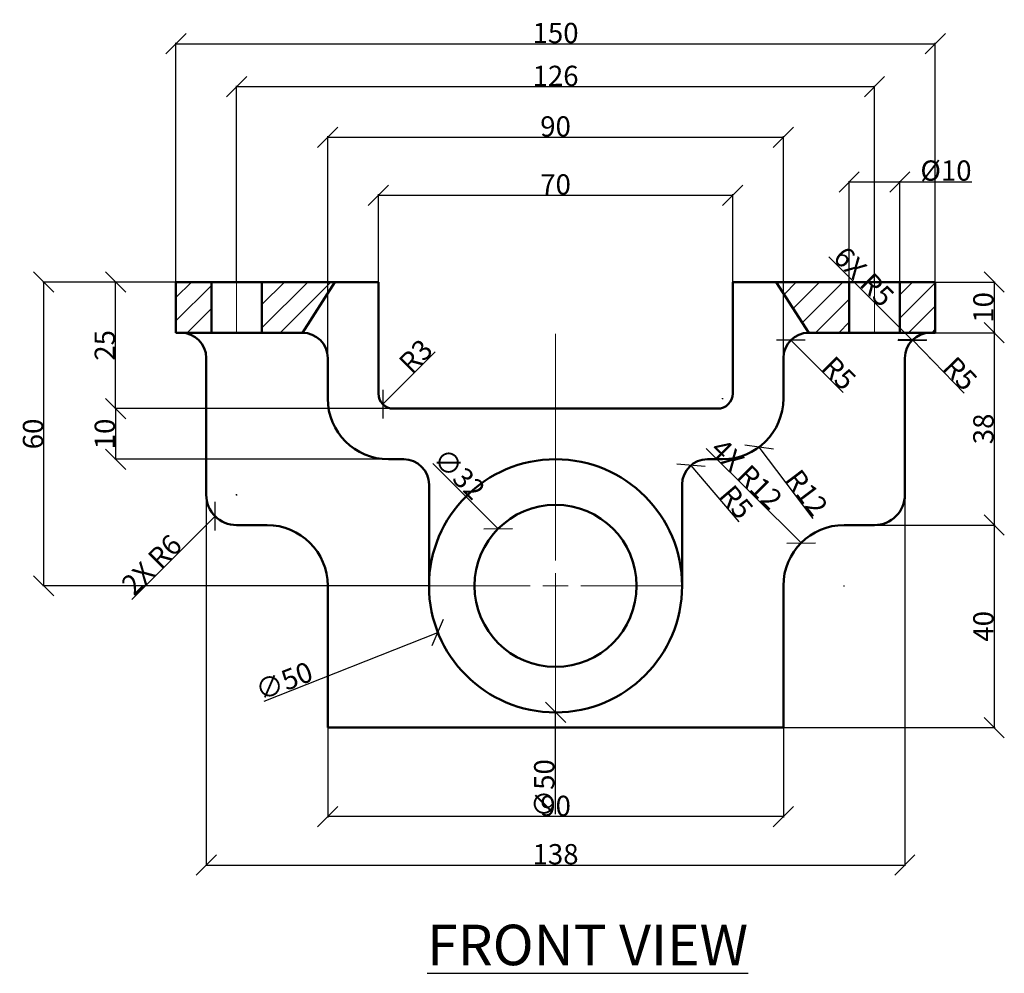
# Model space of a CAD drawing. Units: millimetres. Extents: x 113 to 503, y 39 to 409.
# Tile 2 of 3: x 113 to 307, y 221 to 409. Entities that reach past the tile are written whole.
import ezdxf

# ---------------------------------------------------------------- set-up
doc = ezdxf.new("R2010")
doc.units = ezdxf.units.MM
doc.header["$MEASUREMENT"] = 0
doc.linetypes.add('CENTER', pattern=[50.8, 31.75, -6.35, 6.35, -6.35])
for name, color, linetype, lineweight in [('M-CNTR', 1, 'CENTER', 18), ('M-DIMS', 2, 'Continuous', 25), ('M-HATC', 8, 'Continuous', 18), ('M-OUTL', 7, 'Continuous', 50), ('M-TEXT', 3, 'Continuous', 25)]:
    doc.layers.add(name, color=color, linetype=linetype, lineweight=lineweight)
doc.styles.get("Standard").update_dxf_attribs({"font": 'arial.ttf'})
doc.dimstyles.get("Standard").update_dxf_attribs({"dimtxt": 4, "dimasz": 4, "dimexe": 0.18, "dimexo": 0.0625, "dimgap": 0.09, "dimtad": 1, "dimdec": 0, "dimzin": 0, "dimdsep": 46, "dimtxsty": 'Standard', "dimblk": 'OBLIQUE', "dimcen": 0.09, "dimclre": 251, "dimadec": 0, "dimazin": 0, "dimtfac": 1, "dimtdec": 0, "dimtofl": 0, "dimtmove": 0, "dimatfit": 3, "dimfxl": 1, "dimtolj": 1, "dimtzin": 0, "dimarcsym": 0})
pattern_1 = [(45, (99.4996, 254.7123), (-2.298097, 2.298097), [])]

# ---------------------------------------------------------------- blocks, each defined once
blk = doc.blocks.new('*U2')
at = {"layer": 'M-CNTR', "color": 0, "transparency": 16777216}
for p, q in [((0, 5), (0, 25.12)), ((-25.12, 0), (-5, 0)), ((5, 0), (25.12, 0)), ((0, -25.12), (0, -5))]:
    blk.add_line(p, q, dxfattribs=at)
at = {"layer": 'M-CNTR', "color": 0, "linetype": 'Continuous', "transparency": 16777216}
for p, q in [((0, -2.5), (0, 2.5)), ((-2.5, 0), (2.5, 0))]:
    blk.add_line(p, q, dxfattribs=at)
blk = doc.blocks.new('_Oblique')
at = {"color": 0, "linetype": 'ByBlock', "lineweight": -2}
blk.add_line((-0.5, -0.5), (0.5, 0.5), dxfattribs=at)
blk = doc.blocks.new('*D3')
at = {"layer": 'Defpoints', "color": 0, "transparency": 16777216}
for p in [(253.81, 374.39), (183.81, 357.23), (253.81, 357.23)]:
    blk.add_point(p, dxfattribs=at)
at = {"layer": 'M-DIMS', "color": 0, "lineweight": -2, "transparency": 16777216}
for p, q in [((183.81, 357.29), (183.81, 374.57)), ((183.81, 374.39), (253.81, 374.39)), ((253.81, 357.29), (253.81, 374.57))]:
    blk.add_line(p, q, dxfattribs=at)
at = {"layer": 'M-DIMS', "color": 0, "lineweight": -2, "transparency": 16777216, "xscale": 4, "yscale": 4, "zscale": 4, "rotation": 180}
blk.add_blockref('_Oblique', (183.81, 374.39), dxfattribs=at)
at = {"layer": 'M-DIMS', "color": 0, "lineweight": -2, "transparency": 16777216, "xscale": 4, "yscale": 4, "zscale": 4}
blk.add_blockref('_Oblique', (253.81, 374.39), dxfattribs=at)
at = {"layer": 'M-DIMS', "color": 0, "transparency": 16777216, "insert": (218.81, 376.52), "char_height": 4, "attachment_point": 5}
blk.add_mtext('\\A1;70', dxfattribs=at)
blk = doc.blocks.new('*D4')
at = {"layer": 'Defpoints', "color": 0, "transparency": 16777216}
for p in [(263.81, 385.85), (173.81, 342.23), (263.81, 342.23)]:
    blk.add_point(p, dxfattribs=at)
at = {"layer": 'M-DIMS', "color": 0, "lineweight": -2, "transparency": 16777216}
for p, q in [((173.81, 342.29), (173.81, 386.03)), ((173.81, 385.85), (263.81, 385.85)), ((263.81, 342.29), (263.81, 386.03))]:
    blk.add_line(p, q, dxfattribs=at)
at = {"layer": 'M-DIMS', "color": 0, "lineweight": -2, "transparency": 16777216, "xscale": 4, "yscale": 4, "zscale": 4, "rotation": 180}
blk.add_blockref('_Oblique', (173.81, 385.85), dxfattribs=at)
at = {"layer": 'M-DIMS', "color": 0, "lineweight": -2, "transparency": 16777216, "xscale": 4, "yscale": 4, "zscale": 4}
blk.add_blockref('_Oblique', (263.81, 385.85), dxfattribs=at)
at = {"layer": 'M-DIMS', "color": 0, "transparency": 16777216, "insert": (218.81, 387.98), "char_height": 4, "attachment_point": 5}
blk.add_mtext('\\A1;90', dxfattribs=at)
blk = doc.blocks.new('*D5')
at = {"layer": 'Defpoints', "color": 0, "transparency": 16777216}
for p in [(281.81, 395.84), (155.81, 357.23), (281.81, 357.23)]:
    blk.add_point(p, dxfattribs=at)
at = {"layer": 'M-DIMS', "color": 0, "lineweight": -2, "transparency": 16777216}
for p, q in [((155.81, 357.29), (155.81, 396.02)), ((155.81, 395.84), (281.81, 395.84)), ((281.81, 357.29), (281.81, 396.02))]:
    blk.add_line(p, q, dxfattribs=at)
at = {"layer": 'M-DIMS', "color": 0, "lineweight": -2, "transparency": 16777216, "xscale": 4, "yscale": 4, "zscale": 4, "rotation": 180}
blk.add_blockref('_Oblique', (155.81, 395.84), dxfattribs=at)
at = {"layer": 'M-DIMS', "color": 0, "lineweight": -2, "transparency": 16777216, "xscale": 4, "yscale": 4, "zscale": 4}
blk.add_blockref('_Oblique', (281.81, 395.84), dxfattribs=at)
at = {"layer": 'M-DIMS', "color": 0, "transparency": 16777216, "insert": (218.81, 397.97), "char_height": 4, "attachment_point": 5}
blk.add_mtext('\\A1;126', dxfattribs=at)
blk = doc.blocks.new('*D6')
at = {"layer": 'Defpoints', "color": 0, "transparency": 16777216}
for p in [(293.81, 404.31), (143.81, 357.23), (293.81, 357.23)]:
    blk.add_point(p, dxfattribs=at)
at = {"layer": 'M-DIMS', "color": 0, "lineweight": -2, "transparency": 16777216}
for p, q in [((143.81, 357.29), (143.81, 404.49)), ((143.81, 404.31), (293.81, 404.31)), ((293.81, 357.29), (293.81, 404.49))]:
    blk.add_line(p, q, dxfattribs=at)
at = {"layer": 'M-DIMS', "color": 0, "lineweight": -2, "transparency": 16777216, "xscale": 4, "yscale": 4, "zscale": 4, "rotation": 180}
blk.add_blockref('_Oblique', (143.81, 404.31), dxfattribs=at)
at = {"layer": 'M-DIMS', "color": 0, "lineweight": -2, "transparency": 16777216, "xscale": 4, "yscale": 4, "zscale": 4}
blk.add_blockref('_Oblique', (293.81, 404.31), dxfattribs=at)
at = {"layer": 'M-DIMS', "color": 0, "transparency": 16777216, "insert": (218.81, 406.44), "char_height": 4, "attachment_point": 5}
blk.add_mtext('\\A1;150', dxfattribs=at)
blk = doc.blocks.new('*D7')
at = {"layer": 'Defpoints', "color": 0, "transparency": 16777216}
for p in [(286.81, 377.02), (276.81, 357.23), (286.81, 357.23)]:
    blk.add_point(p, dxfattribs=at)
at = {"layer": 'M-DIMS', "color": 0, "lineweight": -2, "transparency": 16777216}
for p, q in [((276.81, 357.29), (276.81, 377.2)), ((276.81, 377.02), (286.81, 377.02)), ((286.81, 357.29), (286.81, 377.2)), ((286.81, 377.02), (301.06, 377.02))]:
    blk.add_line(p, q, dxfattribs=at)
at = {"layer": 'M-DIMS', "color": 0, "lineweight": -2, "transparency": 16777216, "xscale": 4, "yscale": 4, "zscale": 4, "rotation": 180}
blk.add_blockref('_Oblique', (276.81, 377.02), dxfattribs=at)
at = {"layer": 'M-DIMS', "color": 0, "lineweight": -2, "transparency": 16777216, "xscale": 4, "yscale": 4, "zscale": 4}
blk.add_blockref('_Oblique', (286.81, 377.02), dxfattribs=at)
at = {"layer": 'M-DIMS', "color": 0, "transparency": 16777216, "insert": (295.93, 379.26), "char_height": 4, "attachment_point": 5}
blk.add_mtext('\\A1;%%C10', dxfattribs=at)
blk = doc.blocks.new('*D8')
at = {"layer": 'Defpoints', "color": 0, "transparency": 16777216}
for p in [(117.71, 357.23), (143.81, 357.23), (193.69, 297.23)]:
    blk.add_point(p, dxfattribs=at)
at = {"layer": 'M-DIMS', "color": 0, "lineweight": -2, "transparency": 16777216}
for p, q in [((143.75, 357.23), (117.53, 357.23)), ((117.71, 297.23), (117.71, 357.23)), ((193.63, 297.23), (117.53, 297.23))]:
    blk.add_line(p, q, dxfattribs=at)
at = {"layer": 'M-DIMS', "color": 0, "lineweight": -2, "transparency": 16777216, "xscale": 4, "yscale": 4, "zscale": 4}
for p, rotation in [((117.71, 357.23), 90), ((117.71, 297.23), 270)]:
    blk.add_blockref('_Oblique', p, dxfattribs=dict(at, rotation=rotation))
at = {"layer": 'M-DIMS', "color": 0, "transparency": 16777216, "insert": (115.58, 327.23), "char_height": 4, "attachment_point": 5, "rotation": 90}
blk.add_mtext('\\A1;60', dxfattribs=at)
blk = doc.blocks.new('*D9')
at = {"layer": 'Defpoints', "color": 0, "transparency": 16777216}
for p in [(131.9, 357.23), (143.81, 357.23), (186.81, 332.23)]:
    blk.add_point(p, dxfattribs=at)
at = {"layer": 'M-DIMS', "color": 0, "lineweight": -2, "transparency": 16777216}
for p, q in [((143.75, 357.23), (131.72, 357.23)), ((131.9, 332.23), (131.9, 357.23)), ((186.75, 332.23), (131.72, 332.23))]:
    blk.add_line(p, q, dxfattribs=at)
at = {"layer": 'M-DIMS', "color": 0, "lineweight": -2, "transparency": 16777216, "xscale": 4, "yscale": 4, "zscale": 4}
for p, rotation in [((131.9, 357.23), 90), ((131.9, 332.23), 270)]:
    blk.add_blockref('_Oblique', p, dxfattribs=dict(at, rotation=rotation))
at = {"layer": 'M-DIMS', "color": 0, "transparency": 16777216, "insert": (129.76, 344.73), "char_height": 4, "attachment_point": 5, "rotation": 90}
blk.add_mtext('\\A1;25', dxfattribs=at)
blk = doc.blocks.new('*D10')
at = {"layer": 'Defpoints', "color": 0, "transparency": 16777216}
for p in [(186.81, 332.23), (131.9, 322.23), (187.31, 322.23)]:
    blk.add_point(p, dxfattribs=at)
at = {"layer": 'M-DIMS', "color": 0, "lineweight": -2, "transparency": 16777216}
for p, q in [((186.75, 332.23), (131.72, 332.23)), ((131.9, 332.23), (131.9, 322.23)), ((187.25, 322.23), (131.72, 322.23))]:
    blk.add_line(p, q, dxfattribs=at)
at = {"layer": 'M-DIMS', "color": 0, "lineweight": -2, "transparency": 16777216, "xscale": 4, "yscale": 4, "zscale": 4}
for p, rotation in [((131.9, 332.23), 90), ((131.9, 322.23), 270)]:
    blk.add_blockref('_Oblique', p, dxfattribs=dict(at, rotation=rotation))
at = {"layer": 'M-DIMS', "color": 0, "transparency": 16777216, "insert": (129.76, 327.23), "char_height": 4, "attachment_point": 5, "rotation": 90}
blk.add_mtext('\\A1;10', dxfattribs=at)
blk = doc.blocks.new('*D11')
at = {"layer": 'Defpoints', "color": 0, "transparency": 16777216}
for p in [(293.81, 357.23), (293.81, 347.23), (305.46, 347.23)]:
    blk.add_point(p, dxfattribs=at)
at = {"layer": 'M-DIMS', "color": 0, "lineweight": -2, "transparency": 16777216}
for p, q in [((293.87, 357.23), (305.64, 357.23)), ((305.46, 357.23), (305.46, 347.23)), ((293.87, 347.23), (305.64, 347.23))]:
    blk.add_line(p, q, dxfattribs=at)
at = {"layer": 'M-DIMS', "color": 0, "lineweight": -2, "transparency": 16777216, "xscale": 4, "yscale": 4, "zscale": 4}
for p, rotation in [((305.46, 357.23), 90), ((305.46, 347.23), 270)]:
    blk.add_blockref('_Oblique', p, dxfattribs=dict(at, rotation=rotation))
at = {"layer": 'M-DIMS', "color": 0, "transparency": 16777216, "insert": (303.32, 352.23), "char_height": 4, "attachment_point": 5, "rotation": 90}
blk.add_mtext('\\A1;10', dxfattribs=at)
blk = doc.blocks.new('*D12')
at = {"layer": 'Defpoints', "color": 0, "transparency": 16777216}
for p in [(293.81, 347.23), (278.81, 309.23), (305.46, 309.23)]:
    blk.add_point(p, dxfattribs=at)
at = {"layer": 'M-DIMS', "color": 0, "lineweight": -2, "transparency": 16777216}
for p, q in [((293.87, 347.23), (305.64, 347.23)), ((305.46, 347.23), (305.46, 309.23)), ((278.87, 309.23), (305.64, 309.23))]:
    blk.add_line(p, q, dxfattribs=at)
at = {"layer": 'M-DIMS', "color": 0, "lineweight": -2, "transparency": 16777216, "xscale": 4, "yscale": 4, "zscale": 4}
for p, rotation in [((305.46, 347.23), 90), ((305.46, 309.23), 270)]:
    blk.add_blockref('_Oblique', p, dxfattribs=dict(at, rotation=rotation))
at = {"layer": 'M-DIMS', "color": 0, "transparency": 16777216, "insert": (303.32, 328.23), "char_height": 4, "attachment_point": 5, "rotation": 90}
blk.add_mtext('\\A1;38', dxfattribs=at)
blk = doc.blocks.new('*D13')
at = {"layer": 'Defpoints', "color": 0, "transparency": 16777216}
for p in [(278.81, 309.23), (263.81, 269.23), (305.46, 269.23)]:
    blk.add_point(p, dxfattribs=at)
at = {"layer": 'M-DIMS', "color": 0, "lineweight": -2, "transparency": 16777216}
for p, q in [((278.87, 309.23), (305.64, 309.23)), ((305.46, 309.23), (305.46, 269.23)), ((263.87, 269.23), (305.64, 269.23))]:
    blk.add_line(p, q, dxfattribs=at)
at = {"layer": 'M-DIMS', "color": 0, "lineweight": -2, "transparency": 16777216, "xscale": 4, "yscale": 4, "zscale": 4}
for p, rotation in [((305.46, 309.23), 90), ((305.46, 269.23), 270)]:
    blk.add_blockref('_Oblique', p, dxfattribs=dict(at, rotation=rotation))
at = {"layer": 'M-DIMS', "color": 0, "transparency": 16777216, "insert": (303.32, 289.23), "char_height": 4, "attachment_point": 5, "rotation": 90}
blk.add_mtext('\\A1;40', dxfattribs=at)
blk = doc.blocks.new('*D14')
at = {"layer": 'Defpoints', "color": 0, "transparency": 16777216}
for p in [(173.81, 269.23), (263.81, 269.23), (173.81, 251.63)]:
    blk.add_point(p, dxfattribs=at)
at = {"layer": 'M-DIMS', "color": 0, "lineweight": -2, "transparency": 16777216}
for p, q in [((173.81, 269.16), (173.81, 251.45)), ((263.81, 269.16), (263.81, 251.45)), ((263.81, 251.63), (173.81, 251.63))]:
    blk.add_line(p, q, dxfattribs=at)
at = {"layer": 'M-DIMS', "color": 0, "lineweight": -2, "transparency": 16777216, "xscale": 4, "yscale": 4, "zscale": 4, "rotation": 180}
blk.add_blockref('_Oblique', (173.81, 251.63), dxfattribs=at)
at = {"layer": 'M-DIMS', "color": 0, "lineweight": -2, "transparency": 16777216, "xscale": 4, "yscale": 4, "zscale": 4}
blk.add_blockref('_Oblique', (263.81, 251.63), dxfattribs=at)
at = {"layer": 'M-DIMS', "color": 0, "transparency": 16777216, "insert": (218.81, 253.76), "char_height": 4, "attachment_point": 5}
blk.add_mtext('\\A1;90', dxfattribs=at)
blk = doc.blocks.new('*D15')
at = {"layer": 'Defpoints', "color": 0, "transparency": 16777216}
for p in [(149.81, 315.23), (287.81, 315.23), (287.81, 242.08)]:
    blk.add_point(p, dxfattribs=at)
at = {"layer": 'M-DIMS', "color": 0, "lineweight": -2, "transparency": 16777216}
for p, q in [((149.81, 315.16), (149.81, 241.9)), ((287.81, 315.16), (287.81, 241.9)), ((149.81, 242.08), (287.81, 242.08))]:
    blk.add_line(p, q, dxfattribs=at)
at = {"layer": 'M-DIMS', "color": 0, "lineweight": -2, "transparency": 16777216, "xscale": 4, "yscale": 4, "zscale": 4, "rotation": 180}
blk.add_blockref('_Oblique', (149.81, 242.08), dxfattribs=at)
at = {"layer": 'M-DIMS', "color": 0, "lineweight": -2, "transparency": 16777216, "xscale": 4, "yscale": 4, "zscale": 4}
blk.add_blockref('_Oblique', (287.81, 242.08), dxfattribs=at)
at = {"layer": 'M-DIMS', "color": 0, "transparency": 16777216, "insert": (218.81, 244.21), "char_height": 4, "attachment_point": 5}
blk.add_mtext('\\A1;138', dxfattribs=at)
blk = doc.blocks.new('*D16')
at = {"layer": 'Defpoints', "color": 0, "transparency": 16777216}
for p in [(242.06, 306.42), (195.56, 288.03)]:
    blk.add_point(p, dxfattribs=at)
at = {"layer": 'M-DIMS', "color": 0, "lineweight": -2, "transparency": 16777216}
for p, q in [((218.72, 297.23), (218.9, 297.23)), ((218.81, 297.14), (218.81, 297.32)), ((161.23, 274.45), (195.56, 288.03))]:
    blk.add_line(p, q, dxfattribs=at)
at = {"layer": 'M-DIMS', "color": 0, "lineweight": -2, "transparency": 16777216, "xscale": 4, "yscale": 4, "zscale": 4, "rotation": 21.58340125871024}
blk.add_blockref('_Oblique', (195.56, 288.03), dxfattribs=at)
at = {"layer": 'M-DIMS', "color": 0, "transparency": 16777216, "insert": (165.17, 278.42), "char_height": 4, "attachment_point": 5, "rotation": 21.5834}
blk.add_mtext('\\A1;∅50', dxfattribs=at)
blk = doc.blocks.new('*D17')
at = {"layer": 'Defpoints', "color": 0, "transparency": 16777216}
for p in [(186.81, 335.23), (184.69, 333.11)]:
    blk.add_point(p, dxfattribs=at)
at = {"layer": 'M-DIMS', "color": 0, "lineweight": -2, "transparency": 16777216}
blk.add_line((195.03, 343.45), (184.69, 333.11), dxfattribs=at)
at = {"layer": 'M-DIMS', "color": 0, "lineweight": -2, "transparency": 16777216, "xscale": 4, "yscale": 4, "zscale": 4, "rotation": 224.9999999999992}
blk.add_blockref('_Oblique', (184.69, 333.11), dxfattribs=at)
at = {"layer": 'M-DIMS', "color": 0, "transparency": 16777216, "insert": (191.18, 342.62), "char_height": 4, "attachment_point": 5, "rotation": 45}
blk.add_mtext('\\A1;R3', dxfattribs=at)
blk = doc.blocks.new('*D18')
at = {"layer": 'Defpoints', "color": 0, "transparency": 16777216}
for p in [(251.81, 334.23), (259.03, 324.64)]:
    blk.add_point(p, dxfattribs=at)
at = {"layer": 'M-DIMS', "color": 0, "lineweight": -2, "transparency": 16777216}
for p, q in [((251.72, 334.23), (251.9, 334.23)), ((251.81, 334.14), (251.81, 334.32)), ((269.67, 310.5), (259.03, 324.64))]:
    blk.add_line(p, q, dxfattribs=at)
at = {"layer": 'M-DIMS', "color": 0, "lineweight": -2, "transparency": 16777216, "xscale": 4, "yscale": 4, "zscale": 4, "rotation": 126.9814045897615}
blk.add_blockref('_Oblique', (259.03, 324.64), dxfattribs=at)
at = {"layer": 'M-DIMS', "color": 0, "transparency": 16777216, "insert": (268.43, 315.64), "char_height": 4, "attachment_point": 5, "rotation": 306.9814}
blk.add_mtext('\\A1;R12', dxfattribs=at)
blk = doc.blocks.new('*D19')
at = {"layer": 'Defpoints', "color": 0, "transparency": 16777216}
for p in [(265.27, 345.76), (268.81, 342.23)]:
    blk.add_point(p, dxfattribs=at)
at = {"layer": 'M-DIMS', "color": 0, "lineweight": -2, "transparency": 16777216}
blk.add_line((275.64, 335.4), (265.27, 345.76), dxfattribs=at)
at = {"layer": 'M-DIMS', "color": 0, "lineweight": -2, "transparency": 16777216, "xscale": 4, "yscale": 4, "zscale": 4, "rotation": 135}
blk.add_blockref('_Oblique', (265.27, 345.76), dxfattribs=at)
at = {"layer": 'M-DIMS', "color": 0, "transparency": 16777216, "insert": (274.79, 339.25), "char_height": 4, "attachment_point": 5, "rotation": 315}
blk.add_mtext('\\A1;R5', dxfattribs=at)
blk = doc.blocks.new('*D20')
at = {"layer": 'Defpoints', "color": 0, "transparency": 16777216}
for p in [(245.57, 321.03), (248.81, 317.23)]:
    blk.add_point(p, dxfattribs=at)
at = {"layer": 'M-DIMS', "color": 0, "lineweight": -2, "transparency": 16777216}
blk.add_line((255.08, 309.87), (245.57, 321.03), dxfattribs=at)
at = {"layer": 'M-DIMS', "color": 0, "lineweight": -2, "transparency": 16777216, "xscale": 4, "yscale": 4, "zscale": 4, "rotation": 130.4320205040033}
blk.add_blockref('_Oblique', (245.57, 321.03), dxfattribs=at)
at = {"layer": 'M-DIMS', "color": 0, "transparency": 16777216, "insert": (254.53, 313.79), "char_height": 4, "attachment_point": 5, "rotation": 310.432}
blk.add_mtext('\\A1;R5', dxfattribs=at)
blk = doc.blocks.new('*D21')
at = {"layer": 'Defpoints', "color": 0, "transparency": 16777216}
for p in [(289.33, 345.82), (292.81, 342.23)]:
    blk.add_point(p, dxfattribs=at)
at = {"layer": 'M-DIMS', "color": 0, "lineweight": -2, "transparency": 16777216}
blk.add_line((299.53, 335.29), (289.33, 345.82), dxfattribs=at)
at = {"layer": 'M-DIMS', "color": 0, "lineweight": -2, "transparency": 16777216, "xscale": 4, "yscale": 4, "zscale": 4, "rotation": 134.0656680550646}
blk.add_blockref('_Oblique', (289.33, 345.82), dxfattribs=at)
at = {"layer": 'M-DIMS', "color": 0, "transparency": 16777216, "insert": (298.74, 339.16), "char_height": 4, "attachment_point": 5, "rotation": 314.0657}
blk.add_mtext('\\A1;R5', dxfattribs=at)
blk = doc.blocks.new('*D49')
at = {"layer": 'Defpoints', "color": 0, "transparency": 16777216}
for p in [(218.81, 322.23), (218.81, 272.23)]:
    blk.add_point(p, dxfattribs=at)
at = {"layer": 'M-DIMS', "color": 251, "lineweight": -2, "transparency": 16777216}
for p, q in [((218.72, 297.23), (218.9, 297.23)), ((218.81, 297.14), (218.81, 297.32))]:
    blk.add_line(p, q, dxfattribs=at)
at = {"layer": 'M-DIMS', "color": 0, "lineweight": -2, "transparency": 16777216}
blk.add_line((218.81, 252.1), (218.81, 272.23), dxfattribs=at)
at = {"layer": 'M-DIMS', "color": 0, "lineweight": -2, "transparency": 16777216, "xscale": 4, "yscale": 4, "zscale": 4, "rotation": 89.9994591278414}
blk.add_blockref('_Oblique', (218.81, 272.23), dxfattribs=at)
at = {"layer": 'M-DIMS', "color": 0, "transparency": 16777216, "insert": (216.57, 257.23), "char_height": 4, "attachment_point": 5, "rotation": 89.9995}
blk.add_mtext('\\A1;∅50', dxfattribs=at)
blk = doc.blocks.new('*D50')
at = {"layer": 'Defpoints', "color": 0, "transparency": 16777216}
for p in [(207.48, 308.52), (230.14, 285.93)]:
    blk.add_point(p, dxfattribs=at)
at = {"layer": 'M-DIMS', "color": 0, "lineweight": -2, "transparency": 16777216}
blk.add_line((194.57, 321.38), (207.48, 308.52), dxfattribs=at)
at = {"layer": 'M-DIMS', "color": 251, "lineweight": -2, "transparency": 16777216}
for p, q in [((218.72, 297.23), (218.9, 297.23)), ((218.81, 297.14), (218.81, 297.32))]:
    blk.add_line(p, q, dxfattribs=at)
at = {"layer": 'M-DIMS', "color": 0, "lineweight": -2, "transparency": 16777216, "xscale": 4, "yscale": 4, "zscale": 4, "rotation": 315.0941070098264}
blk.add_blockref('_Oblique', (207.48, 308.52), dxfattribs=at)
at = {"layer": 'M-DIMS', "color": 0, "transparency": 16777216, "insert": (199.78, 319.37), "char_height": 4, "attachment_point": 5, "rotation": 315.0941}
blk.add_mtext('\\A1;∅32', dxfattribs=at)
blk = doc.blocks.new('*D51')
at = {"layer": 'Defpoints', "color": 0, "transparency": 16777216}
for p in [(267.31, 305.69), (275.81, 297.23)]:
    blk.add_point(p, dxfattribs=at)
at = {"layer": 'M-DIMS', "color": 0, "lineweight": -2, "transparency": 16777216}
blk.add_line((248.56, 324.36), (267.31, 305.69), dxfattribs=at)
at = {"layer": 'M-DIMS', "color": 251, "lineweight": -2, "transparency": 16777216}
for p, q in [((275.72, 297.23), (275.9, 297.23)), ((275.81, 297.14), (275.81, 297.32))]:
    blk.add_line(p, q, dxfattribs=at)
at = {"layer": 'M-DIMS', "color": 0, "lineweight": -2, "transparency": 16777216, "xscale": 4, "yscale": 4, "zscale": 4, "rotation": 315.1251384350903}
blk.add_blockref('_Oblique', (267.31, 305.69), dxfattribs=at)
at = {"layer": 'M-DIMS', "color": 0, "transparency": 16777216, "insert": (256.58, 319.34), "char_height": 4, "attachment_point": 5, "rotation": 315.1251}
blk.add_mtext('\\A1;4X R12', dxfattribs=at)
blk = doc.blocks.new('*D52')
at = {"layer": 'Defpoints', "color": 0, "transparency": 16777216}
for p in [(289.27, 345.76), (292.81, 342.23)]:
    blk.add_point(p, dxfattribs=at)
at = {"layer": 'M-DIMS', "color": 0, "lineweight": -2, "transparency": 16777216}
blk.add_line((272.82, 362.22), (289.27, 345.76), dxfattribs=at)
at = {"layer": 'M-DIMS', "color": 251, "lineweight": -2, "transparency": 16777216}
for p, q in [((292.72, 342.23), (292.9, 342.23)), ((292.81, 342.14), (292.81, 342.32))]:
    blk.add_line(p, q, dxfattribs=at)
at = {"layer": 'M-DIMS', "color": 0, "lineweight": -2, "transparency": 16777216, "xscale": 4, "yscale": 4, "zscale": 4, "rotation": 315.000753564843}
blk.add_blockref('_Oblique', (289.27, 345.76), dxfattribs=at)
at = {"layer": 'M-DIMS', "color": 0, "transparency": 16777216, "insert": (279.72, 358.33), "char_height": 4, "attachment_point": 5, "rotation": 315.0008}
blk.add_mtext('\\A1;6X R5', dxfattribs=at)
blk = doc.blocks.new('*D53')
at = {"layer": 'Defpoints', "color": 0, "transparency": 16777216}
for p in [(155.81, 315.23), (151.57, 310.98)]:
    blk.add_point(p, dxfattribs=at)
at = {"layer": 'M-DIMS', "color": 251, "lineweight": -2, "transparency": 16777216}
for p, q in [((155.72, 315.23), (155.9, 315.23)), ((155.81, 315.14), (155.81, 315.32))]:
    blk.add_line(p, q, dxfattribs=at)
at = {"layer": 'M-DIMS', "color": 0, "lineweight": -2, "transparency": 16777216}
blk.add_line((135.1, 294.51), (151.57, 310.98), dxfattribs=at)
at = {"layer": 'M-DIMS', "color": 0, "lineweight": -2, "transparency": 16777216, "xscale": 4, "yscale": 4, "zscale": 4, "rotation": 45.00419322341977}
blk.add_blockref('_Oblique', (151.57, 310.98), dxfattribs=at)
at = {"layer": 'M-DIMS', "color": 0, "transparency": 16777216, "insert": (139, 301.43), "char_height": 4, "attachment_point": 5, "rotation": 45.0042}
blk.add_mtext('\\A1;2X R6', dxfattribs=at)

msp = doc.modelspace()

# ---------------------------------------------------------------- hatches: boundary and pattern name
at = {"layer": 'M-HATC'}
h = msp.add_hatch(dxfattribs=at)
h.set_pattern_fill('ANSI31', color=256, scale=26)
h.set_pattern_definition(pattern_1)
h.paths.add_polyline_path([(143.81, 347.227), (150.81, 347.227), (150.81, 357.227), (143.81, 357.227)])
h.paths.add_polyline_path([(286.81, 347.227), (293.81, 347.227), (293.81, 357.227), (286.81, 357.227)])
h = msp.add_hatch(dxfattribs=at)
h.set_pattern_fill('ANSI31', color=256, scale=26)
h.set_pattern_definition(pattern_1)
h.paths.add_polyline_path([(175.235, 357.227), (160.81, 357.227), (160.81, 347.227), (168.81, 347.227)])
h.paths.add_polyline_path([(276.81, 357.227), (262.386, 357.227), (268.81, 347.227), (276.81, 347.227)])

# ---------------------------------------------------------------- linework, layer by layer
at = {"layer": 'M-CNTR'}
for p, q in [((155.81, 347.227), (155.81, 357.227)), ((281.81, 357.227), (281.81, 347.227)), ((218.81, 347.021), (218.81, 260.421))]:
    msp.add_line(p, q, dxfattribs=at)
at = {"layer": 'M-OUTL'}
for p, q in [((183.81, 357.227), (143.81, 357.227)), ((143.81, 347.227), (143.81, 357.227)), ((150.81, 347.227), (150.81, 357.227)), ((160.81, 347.227), (160.81, 357.227)), ((168.81, 347.227), (175.235, 357.227)), ((183.81, 335.227), (183.81, 357.227)), ((253.81, 335.227), (253.81, 357.227)), ((253.81, 357.227), (293.81, 357.227)), ((268.81, 347.227), (262.386, 357.227)), ((276.81, 357.227), (276.81, 347.227)), ((286.81, 357.227), (286.81, 347.227)), ((293.81, 347.227), (293.81, 357.227)), ((168.81, 347.227), (143.81, 347.227)), ((268.81, 347.227), (293.81, 347.227)), ((149.81, 315.227), (149.81, 342.227)), ((173.81, 342.227), (173.81, 334.227)), ((173.81, 342.227), (173.81, 334.227)), ((263.81, 342.227), (263.81, 334.227)), ((263.81, 334.227), (263.81, 342.227)), ((287.81, 315.227), (287.81, 342.227)), ((186.81, 332.227), (250.81, 332.227)), ((185.81, 322.227), (188.81, 322.227)), ((248.81, 322.227), (251.81, 322.227)), ((193.81, 297.227), (193.81, 317.227)), ((243.81, 297.227), (243.81, 317.227)), ((161.81, 309.227), (155.81, 309.227)), ((275.81, 309.227), (281.81, 309.227)), ((173.81, 297.227), (173.81, 269.227)), ((263.81, 297.227), (263.81, 269.227)), ((173.81, 269.227), (263.81, 269.227))]:
    msp.add_line(p, q, dxfattribs=at)
for radius in [25, 16]:
    msp.add_circle((218.81, 297.227), radius, dxfattribs=at)
for centre, radius, start, end in [((144.81, 342.227), 5, 0, 90), ((168.81, 342.227), 5, 0, 90), ((268.81, 342.227), 5, 90, 180), ((292.81, 342.227), 5, 90, 180), ((186.81, 335.227), 3, 180, 270), ((250.81, 335.227), 3, 270, 0), ((185.81, 334.227), 12, 180, 270), ((251.81, 334.227), 12, 270, 0), ((188.81, 317.227), 5, 0, 90), ((248.81, 317.227), 5, 90, 180), ((155.81, 315.227), 6, 180, 270), ((281.81, 315.227), 6, 270, 0), ((161.81, 297.227), 12, 0, 90), ((275.81, 297.227), 12, 90, 180)]:
    msp.add_arc(centre, radius, start, end, dxfattribs=at)

# ---------------------------------------------------------------- block references
at = {"layer": 'M-CNTR'}
msp.add_blockref('*U2', (218.81, 297.227), dxfattribs=at)

# ---------------------------------------------------------------- texts
at = {"layer": 'M-TEXT', "ltscale": 5, "insert": (193.436, 230.285), "char_height": 8, "attachment_point": 1}
msp.add_mtext_dynamic_manual_height_columns('{\\LFRONT VIEW}', width=109.02237, gutter_width=1, heights=[0], dxfattribs=at)

# ---------------------------------------------------------------- dimensions: what is measured, and where the dimension line sits
at = {"layer": 'M-DIMS'}
for base, p1, p2, picture, middle in [((293.81, 404.309), (143.81, 357.227), (293.81, 357.227), '*D6', (218.81, 406.441)), ((281.81, 395.841), (155.81, 357.227), (281.81, 357.227), '*D5', (218.81, 397.973)), ((263.81, 385.847), (173.81, 342.227), (263.81, 342.227), '*D4', (218.81, 387.98)), ((253.81, 374.388), (183.81, 357.227), (253.81, 357.227), '*D3', (218.81, 376.521)), ((287.81, 242.08), (149.81, 315.227), (287.81, 315.227), '*D15', (218.81, 244.214)), ((173.81, 251.631), (263.81, 269.227), (173.81, 269.227), '*D14', (218.81, 253.763))]:
    dim = msp.add_linear_dim(base=base, p1=p1, p2=p2, dimstyle='Standard', override={"dimclrd": 0, "dimclre": 0, "dimclrt": 0}, dxfattribs=at)
    dim.commit()
    dim.dimension.update_dxf_attribs({"geometry": picture, "text_midpoint": middle})
dim = msp.add_linear_dim(base=(286.81, 377.016), p1=(276.81, 357.227), p2=(286.81, 357.227), text='%%C<>', dimstyle='Standard', override={"dimclrd": 0, "dimclre": 0, "dimclrt": 0}, dxfattribs=at)
dim.commit()
dim.dimension.update_dxf_attribs({"geometry": '*D7', "text_midpoint": (295.934, 379.26)})
for center, mpoint, text, picture, middle in [((292.81, 342.227), (289.275, 345.762), '6X <>', '*D52', (279.724, 358.328)), ((275.81, 297.227), (267.306, 305.694), '4X <>', '*D51', (256.58, 319.336)), ((155.81, 315.227), (151.568, 310.984), '2X <>', '*D53', (138.998, 301.428))]:
    dim = msp.add_radius_dim(center=center, mpoint=mpoint, text=text, dimstyle='Standard', override={"dimdec": 0, "dimlfac": 1, "dimrnd": 0, "dimzin": 0, "dimdsep": 46, "dimlunit": 2}, dxfattribs=at)
    dim.commit()
    dim.dimension.update_dxf_attribs({"geometry": picture, "text_midpoint": middle})
for base, p1, p2, picture, middle in [((117.71, 357.227), (193.69, 297.227), (143.81, 357.227), '*D8', (115.578, 327.227)), ((131.897, 357.227), (186.81, 332.227), (143.81, 357.227), '*D9', (129.764, 344.727)), ((305.455, 347.227), (293.81, 357.227), (293.81, 347.227), '*D11', (303.323, 352.227)), ((305.455, 309.227), (293.81, 347.227), (278.81, 309.227), '*D12', (303.322, 328.227)), ((131.897, 322.227), (186.81, 332.227), (187.31, 322.227), '*D10', (129.764, 327.227)), ((305.455, 269.227), (278.81, 309.227), (263.81, 269.227), '*D13', (303.323, 289.227))]:
    dim = msp.add_linear_dim(base=base, p1=p1, p2=p2, angle=90, dimstyle='Standard', override={"dimclrd": 0, "dimclre": 0, "dimclrt": 0}, dxfattribs=at)
    dim.commit()
    dim.dimension.update_dxf_attribs({"geometry": picture, "text_midpoint": middle})
for center, mpoint, picture, middle in [((186.81, 335.227), (184.689, 333.106), '*D17', (192.69, 341.107)), ((268.81, 342.227), (265.275, 345.762), '*D19', (273.286, 337.751)), ((292.81, 342.227), (289.333, 345.82), '*D21', (297.213, 337.678)), ((248.81, 317.227), (245.568, 321.033), '*D20', (252.916, 312.409))]:
    dim = msp.add_radius_dim(center=center, mpoint=mpoint, dimstyle='Standard', override={"dimclrd": 0, "dimclre": 0, "dimclrt": 0}, dxfattribs=at)
    dim.commit()
    dim.dimension.update_dxf_attribs({"geometry": picture, "text_midpoint": middle, "dimtype": 164})
dim = msp.add_radius_dim(center=(251.81, 334.227), mpoint=(259.029, 324.641), dimstyle='Standard', override={"dimclrd": 0, "dimclre": 0, "dimclrt": 0}, dxfattribs=at)
dim.commit()
dim.dimension.update_dxf_attribs({"geometry": '*D18', "text_midpoint": (268.434, 315.639)})
for p1, p2, override, picture, middle in [((230.143, 285.932), (207.478, 308.522), {"dimdec": 0, "dimlfac": 1, "dimrnd": 0, "dimzin": 0, "dimdsep": 46, "dimlunit": 2}, '*D50', (198.192, 317.777)), ((218.81, 322.227), (218.81, 272.227), {"dimdec": 0, "dimlfac": 1, "dimrnd": 0, "dimzin": 0, "dimdsep": 46, "dimlunit": 2}, '*D49', (218.81, 257.227)), ((242.057, 306.423), (195.563, 288.03), {"dimclrd": 0, "dimclre": 0, "dimclrt": 0}, '*D16', (165.998, 276.335))]:
    dim = msp.add_diameter_dim_2p(p1=p1, p2=p2, dimstyle='Standard', override=override, dxfattribs=at)
    dim.commit()
    dim.dimension.update_dxf_attribs({"geometry": picture, "text_midpoint": middle, "dimtype": 163})

doc.saveas('drawing.dxf')
